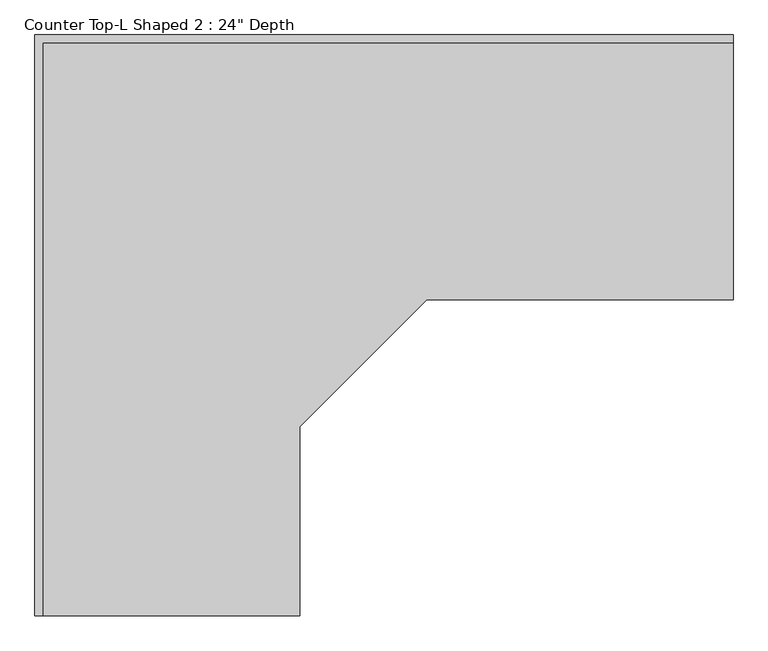
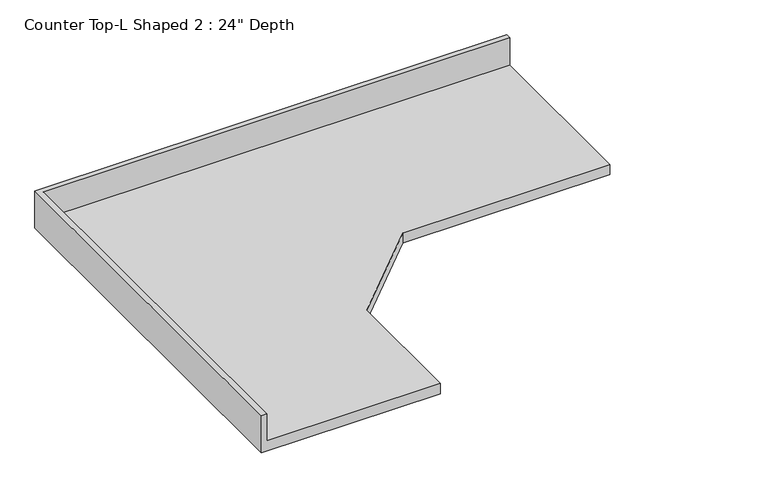
"""IFC4 building model written with IfcOpenShell, lengths in millimetres: furniture geometry."""

from ifc_helpers import new_model, si_unit, origin, place, context, project, spatial, faceted_brep, source, transform, mapped, element, save


def furniture_96954d7a(model_context):
    return source(origin(), model_context, "Body", "Brep", [
        faceted_brep([(-565.4622951, -1392.6224424, 914.4), (-565.4622951, -939.8, 914.4), (-260.6622951, -635.0, 914.4), (473.618312, -635.0, 914.4), (473.618312, -19.05, 914.4), (-1181.4122951, -19.05, 914.4), (-1181.4122951, -1392.6224424, 914.4), (473.618312, 0.0, 876.3), (473.618312, -635.0, 876.3), (-260.6622951, -635.0, 876.3), (-565.4622951, -939.8, 876.3), (-565.4622951, -1392.6224424, 876.3), (-1200.4622951, -1392.6224424, 876.3), (-1200.4622951, 0.0, 876.3), (-1200.4622951, 0.0, 1016.0), (473.618312, 0.0, 1016.0), (-1200.4622951, -1392.6224424, 1016.0), (-1181.4122951, -1392.6224424, 1016.0), (473.618312, -19.05, 1016.0), (-1181.4122951, -19.05, 1016.0)], [[[0, 1, 2, 3, 4, 5, 6]], [[7, 8, 9, 10, 11, 12, 13]], [[7, 13, 14, 15]], [[13, 12, 16, 14]], [[16, 12, 11, 0, 6, 17]], [[1, 0, 11, 10]], [[2, 1, 10, 9]], [[3, 2, 9, 8]], [[8, 7, 15, 18, 4, 3]], [[14, 16, 17, 19, 18, 15]], [[4, 18, 19, 5]], [[19, 17, 6, 5]]]),
    ])


if __name__ == "__main__":
    model = new_model("IFC4")
    model_context = context("Model", 3, world=origin())
    ifc_project = project(units=[si_unit("LENGTHUNIT", "METRE", prefix="MILLI")], contexts=[model_context])
    site = spatial("IfcSite", under=ifc_project)
    building = spatial("IfcBuilding", under=site)
    placement = place(None, origin())
    furniture_shape = furniture_96954d7a(model_context)
    element("IfcFurniture", 1, ObjectType="Counter Top-L Shaped 2 : 24\" Depth", at=placement, inside=building, context=model_context, shape_type="MappedRepresentation", body=[
        mapped(furniture_shape, transform((0.0, 0.0, 0.0), x_axis=(1.0, 0.0, 0.0), y_axis=(0.0, 1.0, 0.0), z_axis=(0.0, 0.0, 1.0))),
    ])
    save(model, "model.ifc")

# Revit data of these elements
# Type "Counter Top-L Shaped 2 : 24\" Depth"
#   Assembly Code = "C1030400"
#   Counter Thickness = 0' - 1 1/2"
#   Depth = 2' - 1"
#   Height = 3' - 0"
#   Length - Leg 1 [instance default] = 8' - 0"
#   Length - Leg 2 [instance default] = 6' - 0"
#   Counter Top Material = none
#   Default Elevation = 0
# Element 1 (IfcFurniture, "Counter Top-L Shaped 2 : 24\" Depth")
#   Length - Leg 1 = 5' - 5.90869"
#   Length - Leg 2 = 4' - 6.82766"
#   Materials on its faces: "Counter Top"
# Materials
#   "Counter Top": class "Wood", colour RGB 226 177 128, transparency 0
